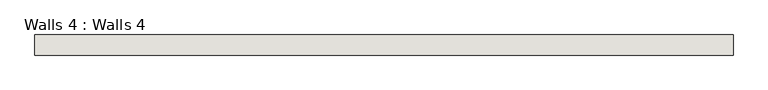
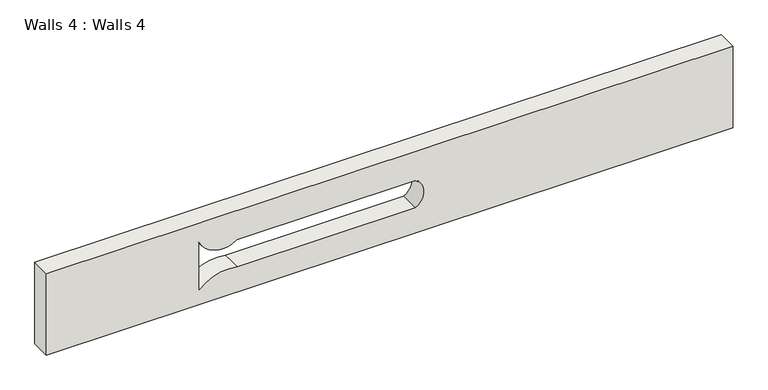
"""IFC4 building model written with IfcOpenShell, lengths in millimetres: wall geometry, Walls 4 : Walls 4."""

from ifc_helpers import new_model, si_unit, point, frame, frame_2d, origin, place, context, project, spatial, polyline, circle_curve, trimmed, segment, composite_curve, outline, extrude, source, transform, mapped, element, save


def walls_4_walls_4_2d9e6e62(model_context):
    return source(origin(), model_context, "Body", "SweptSolid", [
        extrude(outline(polyline([(1323.5671837, 5994.0261575), (1323.5671837, -4569.1738425), (0.0, -4569.1738425), (0.0, 5994.0261575), (1323.5671837, 5994.0261575)]), holes=[composite_curve([segment(polyline([(846.8436691, -1631.4812044), (846.8436691, 1107.0904119)]), True, "CONTINUOUS"), segment(trimmed(circle_curve(frame_2d((629.1536251, 993.3729025)), 245.6025798), [point((846.8436691, 1107.0904119))], [point((411.4635811, 1107.0904119))], True, "CARTESIAN"), True, "CONTINUOUS"), segment(polyline([(411.4635811, 1107.0904119), (411.4635811, -1631.4812044)]), True, "CONTINUOUS"), segment(trimmed(circle_curve(frame_2d((-260.1943618, -1757.5081738)), 683.3792426), [point((411.4635811, -1631.4812044))], [point((242.619759, -2220.3095881))], False, "CARTESIAN"), True, "CONTINUOUS"), segment(polyline([(242.619759, -2220.3095881), (1004.619759, -2220.3095881)]), True, "CONTINUOUS"), segment(trimmed(circle_curve(frame_2d((1176.9737528, -1858.5752949)), 400.6963914), [point((1004.619759, -2220.3095881))], [point((846.8436691, -1631.4812044))], False, "CARTESIAN"), True, "CONTINUOUS")], self_intersect=False)]), frame((0.0, -3443.5510925, 0.0), z_axis=(0.0, 1.0, 0.0), x_axis=(0.0, 0.0, 1.0)), (0.0, 0.0, 1.0), 304.8),
    ])


if __name__ == "__main__":
    model = new_model("IFC4")
    model_context = context("Model", 3, world=origin())
    ifc_project = project(units=[si_unit("LENGTHUNIT", "METRE", prefix="MILLI")], contexts=[model_context])
    site = spatial("IfcSite", under=ifc_project)
    building = spatial("IfcBuilding", under=site)
    placement = place(None, origin())
    walls_4_walls_4_shape = walls_4_walls_4_2d9e6e62(model_context)
    element("IfcWall", 1, ObjectType="Walls 4 : Walls 4", at=placement, inside=building, context=model_context, shape_type="MappedRepresentation", body=[
        mapped(walls_4_walls_4_shape, transform((0.0, 0.0, 0.0), x_axis=(1.0, 0.0, 0.0), y_axis=(0.0, 1.0, 0.0), z_axis=(0.0, 0.0, 1.0))),
    ])
    save(model, "model.ifc")

# Revit data of these elements
# Element 1 (IfcWall, "Walls 4 : Walls 4")
#   Materials on its faces: "Default Wall"
# Materials
#   "Default Wall": colour RGB 80 80 80, transparency 0
